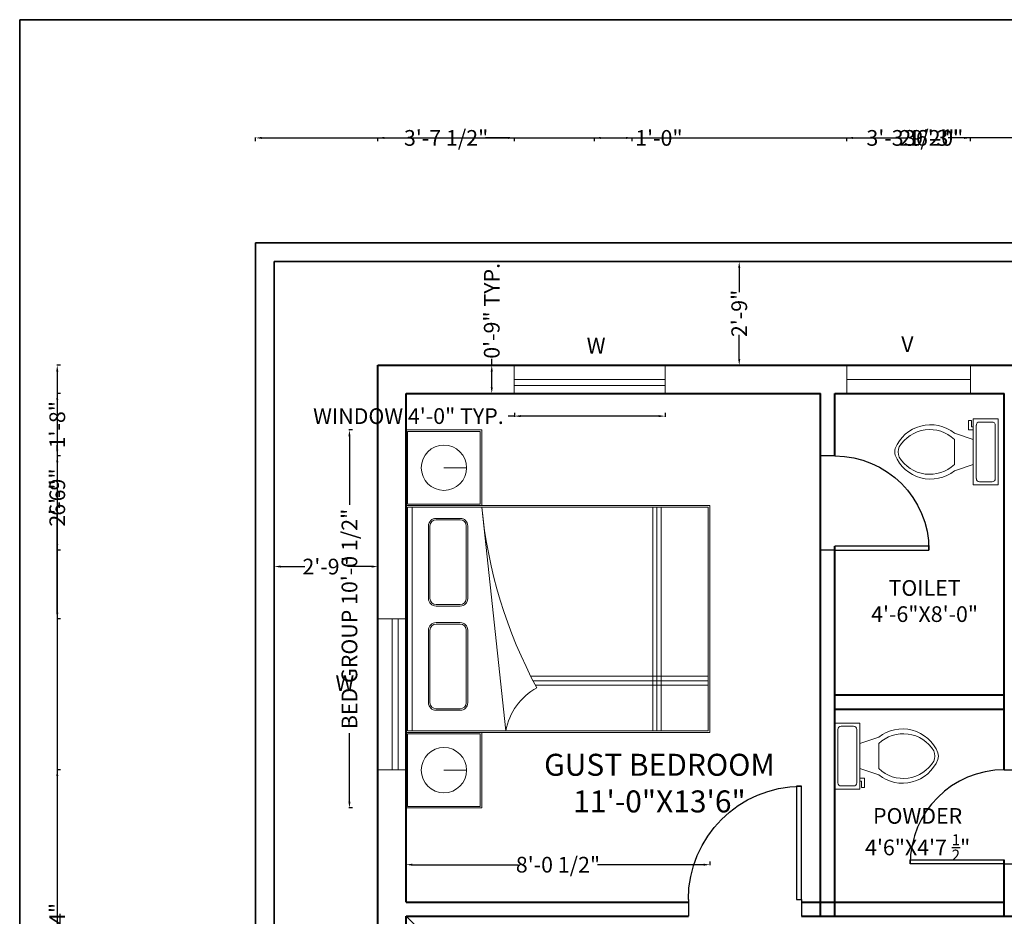
# Model space of a CAD drawing. Units: inches. Extents: x -231 to 349, y -511 to 252.
# Tile 5 of 6: x -231 to 82, y -33 to 252. Entities that reach past the tile are written whole.
import ezdxf

# ---------------------------------------------------------------- set-up
doc = ezdxf.new("R2010")
doc.units = ezdxf.units.IN
doc.header["$MEASUREMENT"] = 0
for name, color, linetype, lineweight in [('A-ANNO-DIMS', 7, 'Continuous', 18), ('A-ANNO-TEXT', 7, 'Continuous', 18), ('A-ANNO-TTLB', 7, 'Continuous', 35), ('A-AREA-IDEN', 7, 'Continuous', 25), ('A-FLOR-FIXT', 8, 'Continuous', 18), ('A-FLOR-STRS', 7, 'Continuous', 20), ('A-GLAZ', 177, 'Continuous', 20), ('A-WALL', 7, 'Continuous', 40), ('BED', 30, 'Continuous', 18), ('C-PROP', 7, 'Continuous', 35), ('DOOR', 42, 'Continuous', 25)]:
    doc.layers.add(name, color=color, linetype=linetype, lineweight=lineweight)
doc.styles.get("Standard").update_dxf_attribs({"font": 'arial.ttf'})
doc.dimstyles.get("Standard").update_dxf_attribs({"dimtxt": 5, "dimasz": 2, "dimexe": 0.18, "dimexo": 0.0625, "dimgap": 0.09, "dimtad": 0, "dimzin": 0, "dimdsep": 46, "dimlunit": 4, "dimtxsty": 'Standard', "dimcen": 0.09, "dimadec": 0, "dimazin": 0, "dimtfac": 1, "dimtofl": 0, "dimtmove": 0, "dimatfit": 3, "dimfxl": 1, "dimfxlon": 1, "dimtolj": 1, "dimtzin": 0, "dimarcsym": 0})

# ---------------------------------------------------------------- blocks, each defined once
blk = doc.blocks.new('*U2')
for p, q in [((0, 0), (0, -6)), ((40, 0), (40, -6))]:
    blk.add_line(p, q)
blk.add_lwpolyline([(0, 0), (0, 40), (1.75, 40), (1.75, 0)], close=True)
blk.add_arc((0, 0), 40, 0, 90)
blk = doc.blocks.new('A$C0EA4476A')
at = {"linetype": 'ByBlock', "lineweight": -2}
for p, q in [((0, 2.008), (0, 1.508)), ((0.5, 2.008), (0, 2.008)), ((0.01, 1.998), (0.01, 1.518)), ((0.49, 1.998), (0.01, 1.998)), ((0.49, 1.518), (0.49, 1.998)), ((0.5, 2.008), (2, 2.008)), ((0.5, 0), (0.5, 2.008)), ((0.5, 1.508), (0.5, 2.008)), ((0.51, 1.998), (1.99, 1.998)), ((0.51, 0.01), (0.51, 1.998)), ((0.51, 1.968), (1.99, 1.968)), ((1.99, 1.998), (1.99, 0.01)), ((2, 2.008), (2, 0)), ((2, 2.008), (2.5, 2.008)), ((2, 1.508), (2, 2.008)), ((2.01, 1.998), (2.49, 1.998)), ((2.01, 1.518), (2.01, 1.998)), ((2.49, 1.998), (2.49, 1.518)), ((2.5, 2.008), (2.5, 1.508)), ((0.696, 1.8603), (1.176, 1.8603)), ((0.696, 1.8503), (1.176, 1.8503)), ((1.3855, 1.8603), (1.8655, 1.8603)), ((1.3855, 1.8503), (1.8655, 1.8503)), ((0.646, 1.6503), (0.646, 1.8103)), ((0.656, 1.6503), (0.656, 1.8103)), ((1.216, 1.8103), (1.216, 1.6503)), ((1.226, 1.8103), (1.226, 1.6503)), ((1.3355, 1.6503), (1.3355, 1.8103)), ((1.3455, 1.6503), (1.3455, 1.8103)), ((1.9055, 1.8103), (1.9055, 1.6503)), ((1.9155, 1.8103), (1.9155, 1.6503)), ((0.25, 1.758), (0.25, 1.608)), ((2.25, 1.758), (2.25, 1.608)), ((1.176, 1.6103), (0.696, 1.6103)), ((1.176, 1.6003), (0.696, 1.6003)), ((1.8655, 1.6103), (1.3855, 1.6103)), ((1.8655, 1.6003), (1.3855, 1.6003)), ((0, 1.508), (0.5, 1.508)), ((0.01, 1.518), (0.49, 1.518)), ((1.99, 1.508), (0.51, 1.3488)), ((2.5, 1.508), (2, 1.508)), ((2.49, 1.518), (2.01, 1.518)), ((0.8715, 1.1845), (0.8715, 0.01)), ((0.8115, 1.1534), (0.8115, 0.01)), ((0.8415, 1.1692), (0.8415, 0.01)), ((0.51, 0.3775), (1.99, 0.3775)), ((0.51, 0.3495), (1.99, 0.3495)), ((0.51, 0.3216), (1.99, 0.3216)), ((1.99, 0.01), (0.51, 0.01)), ((2, 0), (0.5, 0))]:
    blk.add_line(p, q, dxfattribs=at)
for centre in [(0.25, 1.758), (2.25, 1.758)]:
    blk.add_circle(centre, 0.15, dxfattribs=at)
for centre, radius, start, end in [((0.696, 1.8103), 0.05, 90, 180), ((0.696, 1.8103), 0.04, 90, 180), ((1.176, 1.8103), 0.05, 0, 90), ((1.176, 1.8103), 0.04, 0, 90), ((1.3855, 1.8103), 0.05, 90, 180), ((1.3855, 1.8103), 0.04, 90, 180), ((1.8655, 1.8103), 0.05, 0, 90), ((1.8655, 1.8103), 0.04, 0, 90), ((0.696, 1.6503), 0.05, 180, 270), ((0.696, 1.6503), 0.04, 180, 270), ((1.176, 1.6503), 0.04, 270, 0), ((1.176, 1.6503), 0.05, 270, 0), ((1.3855, 1.6503), 0.05, 180, 270), ((1.3855, 1.6503), 0.04, 180, 270), ((1.8655, 1.6503), 0.05, 270, 0), ((1.8655, 1.6503), 0.04, 270, 0), ((2.2933, -1.6357), 3.1583, 95.51042, 118.33991), ((0.4397, 0.9519), 0.4031, 28.46882, 79.95566)]:
    blk.add_arc(centre, radius, start, end, dxfattribs=at)
blk = doc.blocks.new('A$C1A706E3E')
blk.add_blockref('A$C0EA4476A', (0, 0))
blk = doc.blocks.new('*U9')
for p, q in [((9.5, -6), (9.5, -2)), ((-10, -8.5), (-8, -8.5)), ((-10, -9.5), (-10, -8.5)), ((-8, -8.5), (-8, -8)), ((-7, -8), (-7, -9.5)), ((-4, -8), (-6, -14)), ((4, -8), (6, -14)), ((-7, -9.5), (-10, -9.5)), ((4, -14), (-4, -14))]:
    blk.add_line(p, q)
blk.add_lwpolyline([(10.5, -8), (10.5, 0), (-10.5, 0), (-10.5, -8)], close=True)
for points in [[(-9.5, -2), (-9.5, -6)], [(8.5, -1), (-8.5, -1)], [(-8.5, -7), (8.5, -7)]]:
    blk.add_lwpolyline(points)
for centre, radius, start, end in [((-8.62, -1.88), 0.884, 81.8699, 188.1301), ((8.62, -1.88), 0.884, 351.8699, 98.1301), ((-8.62, -6.12), 0.884, 171.8699, 278.1301), ((8.62, -6.12), 0.884, 261.8699, 8.1301), ((3.52, -21.58), 12.17, 141.4691, 247.9714), ((4.2, -21.82), 11.33, 136.3677, 238.9468), ((-3.52, -21.58), 12.17, 292.0284, 38.5307), ((-4.2, -21.82), 11.33, 301.053, 43.6321), ((0, -27.88), 4, 245.7318, 294.2682), ((0, -29), 4, 254.8605, 285.1395)]:
    blk.add_arc(centre, radius, start, end)
blk = doc.blocks.new('*D18')
at = {"layer": 'A-ANNO-DIMS', "color": 0, "lineweight": -2, "transparency": 16777216}
for p, q in [((-150.08, 79.26), (-150.08, 78.08)), ((-117.08, 79.26), (-117.08, 78.08)), ((-148.08, 78.26), (-140.36, 78.26)), ((-119.08, 78.26), (-126.8, 78.26))]:
    blk.add_line(p, q, dxfattribs=at)
at = {"layer": 'A-ANNO-DIMS', "color": 0, "transparency": 16777216}
for points in [[(-148.08, 78.6), (-148.08, 77.93), (-150.08, 78.26)], [(-119.08, 78.6), (-119.08, 77.93), (-117.08, 78.26)]]:
    blk.add_solid(points, dxfattribs=at)
at = {"layer": 'Defpoints', "color": 0, "transparency": 16777216}
for p in [(-150.08, 95.64), (-117.08, 95.64), (-150.08, 78.26)]:
    blk.add_point(p, dxfattribs=at)
at = {"layer": 'A-ANNO-DIMS', "color": 0, "transparency": 16777216, "insert": (-133.58, 78.26), "char_height": 5, "attachment_point": 5}
blk.add_mtext('\\A1;2\'-9"', dxfattribs=at)
blk = doc.blocks.new('*D19')
at = {"layer": 'A-ANNO-DIMS', "color": 0, "lineweight": -2, "transparency": 16777216}
for p, q in [((-2, 175.38), (-2.18, 175.38)), ((-2, 173.38), (-2, 165.66)), ((-2, 144.38), (-2, 152.1)), ((-2, 142.38), (-2.18, 142.38))]:
    blk.add_line(p, q, dxfattribs=at)
at = {"layer": 'A-ANNO-DIMS', "color": 0, "transparency": 16777216}
for points in [[(-2.34, 173.38), (-1.67, 173.38), (-2, 175.38)], [(-2.34, 144.38), (-1.67, 144.38), (-2, 142.38)]]:
    blk.add_solid(points, dxfattribs=at)
at = {"layer": 'Defpoints', "color": 0, "transparency": 16777216}
for p in [(-2, 175.38), (-2, 175.38), (-2, 142.38)]:
    blk.add_point(p, dxfattribs=at)
at = {"layer": 'A-ANNO-DIMS', "color": 0, "transparency": 16777216, "insert": (-2, 158.88), "char_height": 5, "attachment_point": 5, "rotation": 90}
blk.add_mtext('\\A1;2\'-9"', dxfattribs=at)
blk = doc.blocks.new('WIN-48IN')
for p, q in [((224.92, -56.7), (233.92, -56.7)), ((227.42, -56.7), (227.42, -104.7)), ((229.42, -56.7), (229.42, -104.7)), ((224.92, -104.7), (233.92, -104.7))]:
    blk.add_line(p, q)
blk = doc.blocks.new('*D30')
at = {"layer": 'A-ANNO-DIMS', "color": 0, "lineweight": -2, "transparency": 16777216}
for p, q in [((-73.62, 126.18), (-75.62, 126.18)), ((-73.62, 127.18), (-73.62, 126)), ((-27.62, 126.18), (-71.62, 126.18)), ((-25.62, 127.18), (-25.62, 126))]:
    blk.add_line(p, q, dxfattribs=at)
at = {"layer": 'A-ANNO-DIMS', "color": 0, "transparency": 16777216}
for points in [[(-71.62, 126.51), (-71.62, 125.85), (-73.62, 126.18)], [(-27.62, 126.51), (-27.62, 125.85), (-25.62, 126.18)]]:
    blk.add_solid(points, dxfattribs=at)
at = {"layer": 'Defpoints', "color": 0, "transparency": 16777216}
for p in [(-73.62, 133.38), (-25.62, 133.38), (-73.62, 126.18)]:
    blk.add_point(p, dxfattribs=at)
at = {"layer": 'A-ANNO-DIMS', "color": 0, "transparency": 16777216, "insert": (-107.35, 126.18), "char_height": 5, "attachment_point": 5}
blk.add_mtext('\\A1;WINDOW 4\'-0" TYP.', dxfattribs=at)
blk = doc.blocks.new('*D31')
at = {"layer": 'A-ANNO-DIMS', "color": 0, "lineweight": -2, "transparency": 16777216}
for p, q in [((-80.82, 142.38), (-80.82, 144.38)), ((-79.82, 142.38), (-81, 142.38)), ((-80.82, 135.38), (-80.82, 140.38)), ((-79.82, 133.38), (-81, 133.38))]:
    blk.add_line(p, q, dxfattribs=at)
at = {"layer": 'A-ANNO-DIMS', "color": 0, "transparency": 16777216}
for points in [[(-81.16, 140.38), (-80.49, 140.38), (-80.82, 142.38)], [(-81.16, 135.38), (-80.49, 135.38), (-80.82, 133.38)]]:
    blk.add_solid(points, dxfattribs=at)
at = {"layer": 'Defpoints', "color": 0, "transparency": 16777216}
for p in [(-80.82, 142.38), (-73.62, 142.38), (-73.62, 133.38)]:
    blk.add_point(p, dxfattribs=at)
at = {"layer": 'A-ANNO-DIMS', "color": 0, "transparency": 16777216, "insert": (-80.82, 159.71), "char_height": 5, "attachment_point": 5, "rotation": 90}
blk.add_mtext('\\A1;0\'-9" TYP.', dxfattribs=at)
blk = doc.blocks.new('*D34')
at = {"layer": 'A-ANNO-DIMS', "color": 0, "lineweight": -2, "transparency": 16777216}
for p, q in [((-125.14, 121.77), (-126.32, 121.77)), ((-126.14, 119.77), (-126.14, 97.9)), ((-126.14, 3.38), (-126.14, 25.25)), ((-125.14, 1.38), (-126.32, 1.38))]:
    blk.add_line(p, q, dxfattribs=at)
at = {"layer": 'A-ANNO-DIMS', "color": 0, "transparency": 16777216}
for points in [[(-126.47, 119.77), (-125.81, 119.77), (-126.14, 121.77)], [(-126.47, 3.38), (-125.81, 3.38), (-126.14, 1.38)]]:
    blk.add_solid(points, dxfattribs=at)
at = {"layer": 'Defpoints', "color": 0, "transparency": 16777216}
for p in [(-126.14, 121.77), (-108.08, 121.77), (-108.08, 1.38)]:
    blk.add_point(p, dxfattribs=at)
at = {"layer": 'A-ANNO-DIMS', "color": 0, "transparency": 16777216, "insert": (-126.14, 61.57), "char_height": 5, "attachment_point": 5, "rotation": 90}
blk.add_mtext('\\A1;BED GROUP 10\'-0 1/2"', dxfattribs=at)
blk = doc.blocks.new('*D35')
at = {"layer": 'A-ANNO-DIMS', "color": 0, "lineweight": -2, "transparency": 16777216}
for p, q in [((-108.08, -15.68), (-108.08, -16.86)), ((-106.08, -16.68), (-72.29, -16.68)), ((-13.38, -16.68), (-47.16, -16.68)), ((-11.38, -15.68), (-11.38, -16.86))]:
    blk.add_line(p, q, dxfattribs=at)
at = {"layer": 'A-ANNO-DIMS', "color": 0, "transparency": 16777216}
for points in [[(-106.08, -16.35), (-106.08, -17.02), (-108.08, -16.68)], [(-13.38, -16.35), (-13.38, -17.02), (-11.38, -16.68)]]:
    blk.add_solid(points, dxfattribs=at)
at = {"layer": 'Defpoints', "color": 0, "transparency": 16777216}
for p in [(-108.08, 1.38), (-11.38, 1.38), (-108.08, -16.68)]:
    blk.add_point(p, dxfattribs=at)
at = {"layer": 'A-ANNO-DIMS', "color": 0, "transparency": 16777216, "insert": (-59.73, -16.68), "char_height": 5, "attachment_point": 5}
blk.add_mtext('\\A1;8\'-0 1/2"', dxfattribs=at)
blk = doc.blocks.new('*D44')
at = {"layer": 'A-ANNO-DIMS', "color": 0, "lineweight": -2, "transparency": 16777216}
for p, q in [((-156.08, 213.78), (-156.08, 214.96)), ((-154.08, 214.78), (51.24, 214.78)), ((273.92, 214.78), (68.6, 214.78)), ((275.92, 213.78), (275.92, 214.96))]:
    blk.add_line(p, q, dxfattribs=at)
at = {"layer": 'A-ANNO-DIMS', "color": 0, "transparency": 16777216}
for points in [[(-154.08, 215.11), (-154.08, 214.45), (-156.08, 214.78)], [(273.92, 215.11), (273.92, 214.45), (275.92, 214.78)]]:
    blk.add_solid(points, dxfattribs=at)
at = {"layer": 'Defpoints', "color": 0, "transparency": 16777216}
for p in [(275.92, 214.78), (-156.08, 181.38), (275.92, 181.38)]:
    blk.add_point(p, dxfattribs=at)
at = {"layer": 'A-ANNO-DIMS', "color": 0, "transparency": 16777216, "insert": (59.92, 214.78), "char_height": 5, "attachment_point": 5}
blk.add_mtext('\\A1;36\'-0"', dxfattribs=at)
blk = doc.blocks.new('*D46')
at = {"layer": 'A-ANNO-DIMS', "color": 0, "lineweight": -2, "transparency": 16777216}
for p, q in [((-117.08, 213.78), (-117.08, 214.96)), ((-115.08, 214.78), (49.7, 214.78)), ((231.92, 214.78), (67.14, 214.78)), ((233.92, 213.78), (233.92, 214.96))]:
    blk.add_line(p, q, dxfattribs=at)
at = {"layer": 'A-ANNO-DIMS', "color": 0, "transparency": 16777216}
for points in [[(-115.08, 215.11), (-115.08, 214.45), (-117.08, 214.78)], [(231.92, 215.11), (231.92, 214.45), (233.92, 214.78)]]:
    blk.add_solid(points, dxfattribs=at)
at = {"layer": 'Defpoints', "color": 0, "transparency": 16777216}
for p in [(233.92, 214.78), (-117.08, 142.38), (233.92, 142.38)]:
    blk.add_point(p, dxfattribs=at)
at = {"layer": 'A-ANNO-DIMS', "color": 0, "transparency": 16777216, "insert": (58.42, 214.78), "char_height": 5, "attachment_point": 5}
blk.add_mtext('\\A1;29\'-3"', dxfattribs=at)
blk = doc.blocks.new('*D47')
at = {"layer": 'A-ANNO-DIMS', "color": 0, "lineweight": -2, "transparency": 16777216}
for p, q in [((-218.19, 142.38), (-219.37, 142.38)), ((-219.19, 140.38), (-219.19, -87.44)), ((-219.19, -332.62), (-219.19, -104.8)), ((-218.19, -334.62), (-219.37, -334.62))]:
    blk.add_line(p, q, dxfattribs=at)
at = {"layer": 'A-ANNO-DIMS', "color": 0, "transparency": 16777216}
for points in [[(-219.53, 140.38), (-218.86, 140.38), (-219.19, 142.38)], [(-219.53, -332.62), (-218.86, -332.62), (-219.19, -334.62)]]:
    blk.add_solid(points, dxfattribs=at)
at = {"layer": 'Defpoints', "color": 0, "transparency": 16777216}
for p in [(-117.08, 142.38), (-219.19, -334.62), (-96.08, -334.62)]:
    blk.add_point(p, dxfattribs=at)
at = {"layer": 'A-ANNO-DIMS', "color": 0, "transparency": 16777216, "insert": (-219.19, -96.12), "char_height": 5, "attachment_point": 5, "rotation": 90}
blk.add_mtext('\\A1;39\'-9"', dxfattribs=at)
blk = doc.blocks.new('*D49')
at = {"layer": 'A-ANNO-DIMS', "color": 0, "lineweight": -2, "transparency": 16777216}
for p, q in [((-117.08, 213.78), (-117.08, 214.96)), ((-115.08, 214.78), (-107.91, 214.78)), ((-75.62, 214.78), (-82.79, 214.78)), ((-73.62, 213.78), (-73.62, 214.96))]:
    blk.add_line(p, q, dxfattribs=at)
at = {"layer": 'A-ANNO-DIMS', "color": 0, "transparency": 16777216}
for points in [[(-115.08, 215.11), (-115.08, 214.45), (-117.08, 214.78)], [(-75.62, 215.11), (-75.62, 214.45), (-73.62, 214.78)]]:
    blk.add_solid(points, dxfattribs=at)
at = {"layer": 'Defpoints', "color": 0, "transparency": 16777216}
for p in [(-73.62, 214.78), (-117.08, 142.38), (-73.62, 142.38)]:
    blk.add_point(p, dxfattribs=at)
at = {"layer": 'A-ANNO-DIMS', "color": 0, "transparency": 16777216, "insert": (-95.35, 214.78), "char_height": 5, "attachment_point": 5}
blk.add_mtext('\\A1;3\'-7 1/2"', dxfattribs=at)
blk = doc.blocks.new('*D50')
at = {"layer": 'A-ANNO-DIMS', "color": 0, "lineweight": -2, "transparency": 16777216}
for p, q in [((32.24, 213.78), (32.24, 214.96)), ((34.24, 214.78), (39.38, 214.78)), ((69.63, 214.78), (64.49, 214.78)), ((71.63, 213.78), (71.63, 214.96))]:
    blk.add_line(p, q, dxfattribs=at)
at = {"layer": 'A-ANNO-DIMS', "color": 0, "transparency": 16777216}
for points in [[(34.24, 215.11), (34.24, 214.45), (32.24, 214.78)], [(69.63, 215.11), (69.63, 214.45), (71.63, 214.78)]]:
    blk.add_solid(points, dxfattribs=at)
at = {"layer": 'Defpoints', "color": 0, "transparency": 16777216}
for p in [(71.63, 214.78), (32.24, 142.38), (71.63, 142.38)]:
    blk.add_point(p, dxfattribs=at)
at = {"layer": 'A-ANNO-DIMS', "color": 0, "transparency": 16777216, "insert": (51.93, 214.78), "char_height": 5, "attachment_point": 5}
blk.add_mtext('\\A1;3\'-3 1/2"', dxfattribs=at)
blk = doc.blocks.new('*D51')
at = {"layer": 'A-ANNO-DIMS', "color": 0, "lineweight": -2, "transparency": 16777216}
for p, q in [((28.42, -488.55), (28.42, -489.73)), ((32.24, -488.55), (32.24, -489.73)), ((26.42, -489.55), (24.42, -489.55)), ((34.24, -489.55), (36.24, -489.55))]:
    blk.add_line(p, q, dxfattribs=at)
at = {"layer": 'A-ANNO-DIMS', "color": 0, "transparency": 16777216}
for points in [[(26.42, -489.21), (26.42, -489.88), (28.42, -489.55)], [(34.24, -489.21), (34.24, -489.88), (32.24, -489.55)]]:
    blk.add_solid(points, dxfattribs=at)
at = {"layer": 'Defpoints', "color": 0, "transparency": 16777216}
for p in [(28.42, 133.38), (32.24, 133.38), (32.24, -489.55)]:
    blk.add_point(p, dxfattribs=at)
at = {"layer": 'A-ANNO-DIMS', "color": 0, "transparency": 16777216, "insert": (42.97, -489.55), "char_height": 5, "attachment_point": 5}
blk.add_mtext('\\A1;0\'-4"', dxfattribs=at)
blk = doc.blocks.new('*D52')
at = {"layer": 'A-ANNO-DIMS', "color": 0, "lineweight": -2, "transparency": 16777216}
for p, q in [((-218.19, 142.38), (-219.37, 142.38)), ((-219.19, 140.38), (-219.19, 108.73)), ((-219.19, 63.57), (-219.19, 95.23)), ((-218.19, 61.57), (-219.37, 61.57))]:
    blk.add_line(p, q, dxfattribs=at)
at = {"layer": 'A-ANNO-DIMS', "color": 0, "transparency": 16777216}
for points in [[(-219.53, 140.38), (-218.86, 140.38), (-219.19, 142.38)], [(-219.53, 63.57), (-218.86, 63.57), (-219.19, 61.57)]]:
    blk.add_solid(points, dxfattribs=at)
at = {"layer": 'Defpoints', "color": 0, "transparency": 16777216}
for p in [(-117.08, 142.38), (-219.19, 61.57), (-117.08, 61.57)]:
    blk.add_point(p, dxfattribs=at)
at = {"layer": 'A-ANNO-DIMS', "color": 0, "transparency": 16777216, "insert": (-219.19, 101.98), "char_height": 5, "attachment_point": 5, "rotation": 90}
blk.add_mtext('\\A1;6\'-9"', dxfattribs=at)
blk = doc.blocks.new('*D53')
at = {"layer": 'A-ANNO-DIMS', "color": 0, "lineweight": -2, "transparency": 16777216}
for p, q in [((-218.19, 13.57), (-219.37, 13.57)), ((-219.19, 11.57), (-219.19, -29.65)), ((-219.19, -84.36), (-219.19, -43.13)), ((-218.19, -86.36), (-219.37, -86.36))]:
    blk.add_line(p, q, dxfattribs=at)
at = {"layer": 'A-ANNO-DIMS', "color": 0, "transparency": 16777216}
for points in [[(-219.53, 11.57), (-218.86, 11.57), (-219.19, 13.57)], [(-219.53, -84.36), (-218.86, -84.36), (-219.19, -86.36)]]:
    blk.add_solid(points, dxfattribs=at)
at = {"layer": 'Defpoints', "color": 0, "transparency": 16777216}
for p in [(-117.08, 13.57), (-219.19, -86.36), (-117.08, -86.36)]:
    blk.add_point(p, dxfattribs=at)
at = {"layer": 'A-ANNO-DIMS', "color": 0, "transparency": 16777216, "insert": (-219.19, -36.39), "char_height": 5, "attachment_point": 5, "rotation": 90}
blk.add_mtext('\\A1;8\'-4"', dxfattribs=at)
blk = doc.blocks.new('*D59')
at = {"layer": 'A-ANNO-DIMS', "color": 0, "lineweight": -2, "transparency": 16777216}
for p, q in [((17.8, -488.55), (17.8, -489.73)), ((23.92, -488.55), (23.92, -489.73)), ((19.8, -489.55), (21.92, -489.55)), ((23.92, -489.55), (25.92, -489.55))]:
    blk.add_line(p, q, dxfattribs=at)
at = {"layer": 'A-ANNO-DIMS', "color": 0, "transparency": 16777216}
for points in [[(19.8, -489.21), (19.8, -489.88), (17.8, -489.55)], [(21.92, -489.21), (21.92, -489.88), (23.92, -489.55)]]:
    blk.add_solid(points, dxfattribs=at)
at = {"layer": 'Defpoints', "color": 0, "transparency": 16777216}
for p in [(17.8, -28.62), (23.92, -33.12), (23.92, -489.55)]:
    blk.add_point(p, dxfattribs=at)
at = {"layer": 'A-ANNO-DIMS', "color": 0, "transparency": 16777216, "insert": (32.66, -489.55), "char_height": 5, "attachment_point": 5}
blk.add_mtext('\\A1;0\'-6"', dxfattribs=at)
blk = doc.blocks.new('*D61')
at = {"layer": 'A-ANNO-DIMS', "color": 0, "lineweight": -2, "transparency": 16777216}
for p, q in [((-218.19, 113.5), (-219.37, 113.5)), ((-219.19, 111.5), (-219.19, 105.27)), ((-219.19, 85.5), (-219.19, 91.72)), ((-218.19, 83.5), (-219.37, 83.5))]:
    blk.add_line(p, q, dxfattribs=at)
at = {"layer": 'A-ANNO-DIMS', "color": 0, "transparency": 16777216}
for points in [[(-219.53, 111.5), (-218.86, 111.5), (-219.19, 113.5)], [(-219.53, 85.5), (-218.86, 85.5), (-219.19, 83.5)]]:
    blk.add_solid(points, dxfattribs=at)
at = {"layer": 'Defpoints', "color": 0, "transparency": 16777216}
for p in [(28.42, 113.5), (-219.19, 83.5), (28.42, 83.5)]:
    blk.add_point(p, dxfattribs=at)
at = {"layer": 'A-ANNO-DIMS', "color": 0, "transparency": 16777216, "insert": (-219.19, 98.5), "char_height": 5, "attachment_point": 5, "rotation": 90}
blk.add_mtext('\\A1;2\'-6"', dxfattribs=at)
blk = doc.blocks.new('*D62')
at = {"layer": 'A-ANNO-DIMS', "color": 0, "lineweight": -2, "transparency": 16777216}
for p, q in [((-218.19, 133.38), (-219.37, 133.38)), ((-219.19, 131.38), (-219.19, 129.94)), ((-219.19, 115.5), (-219.19, 116.94)), ((-218.19, 113.5), (-219.37, 113.5))]:
    blk.add_line(p, q, dxfattribs=at)
at = {"layer": 'A-ANNO-DIMS', "color": 0, "transparency": 16777216}
for points in [[(-219.53, 131.38), (-218.86, 131.38), (-219.19, 133.38)], [(-219.53, 115.5), (-218.86, 115.5), (-219.19, 113.5)]]:
    blk.add_solid(points, dxfattribs=at)
at = {"layer": 'Defpoints', "color": 0, "transparency": 16777216}
for p in [(28.42, 133.38), (-219.19, 113.5), (28.42, 113.5)]:
    blk.add_point(p, dxfattribs=at)
at = {"layer": 'A-ANNO-DIMS', "color": 0, "transparency": 16777216, "insert": (-219.19, 123.44), "char_height": 5, "attachment_point": 5, "rotation": 90}
blk.add_mtext('\\A1;1\'-8"', dxfattribs=at)
blk = doc.blocks.new('*D68')
at = {"layer": 'A-ANNO-DIMS', "color": 0, "lineweight": -2, "transparency": 16777216}
for p, q in [((-48.08, 213.78), (-48.08, 214.96)), ((-46.08, 214.78), (-38.08, 214.78)), ((-36.08, 213.78), (-36.08, 214.96)), ((-36.08, 214.78), (-34.08, 214.78))]:
    blk.add_line(p, q, dxfattribs=at)
at = {"layer": 'A-ANNO-DIMS', "color": 0, "transparency": 16777216}
for points in [[(-46.08, 215.11), (-46.08, 214.45), (-48.08, 214.78)], [(-38.08, 215.11), (-38.08, 214.45), (-36.08, 214.78)]]:
    blk.add_solid(points, dxfattribs=at)
at = {"layer": 'Defpoints', "color": 0, "transparency": 16777216}
for p in [(-36.08, 214.78), (-48.08, -177.12), (-36.08, -177.12)]:
    blk.add_point(p, dxfattribs=at)
at = {"layer": 'A-ANNO-DIMS', "color": 0, "transparency": 16777216, "insert": (-27.58, 214.78), "char_height": 5, "attachment_point": 5}
blk.add_mtext('\\A1;1\'-0"', dxfattribs=at)

msp = doc.modelspace()

# ---------------------------------------------------------------- linework, layer by layer
at = {"layer": 'A-ANNO-TTLB'}
msp.add_lwpolyline([(-231.158, 252.428), (348.864, 252.428), (348.864, -511.312), (-231.158, -511.312)], close=True, dxfattribs=at)
at = {"layer": 'A-FLOR-STRS'}
msp.add_line((-72.08, -69.12), (-108.08, -33.12), dxfattribs=at)
at = {"layer": 'A-GLAZ'}
for p, q in [((32.236, 142.38), (32.236, 133.38)), ((71.634, 142.38), (71.634, 133.38)), ((71.634, 137.88), (32.236, 137.88))]:
    msp.add_line(p, q, dxfattribs=at)
at = {"layer": 'A-WALL'}
for p, q in [((-117.08, 142.38), (233.92, 142.38)), ((-117.08, -186.12), (-117.08, 142.38)), ((-108.08, 133.38), (23.92, 133.38)), ((-108.08, -28.62), (-108.08, 133.38)), ((23.92, -33.12), (23.92, 133.38)), ((28.42, 133.38), (82.42, 133.38)), ((28.42, 113.495), (28.42, 133.38)), ((82.42, 13.543), (82.42, 133.38)), ((28.42, -33.12), (28.42, 84.808)), ((28.42, 37.38), (82.42, 37.38)), ((28.42, 32.88), (82.42, 32.88)), ((82.42, -33.12), (82.42, -15.145)), ((-108.08, -28.62), (-18.197, -28.62)), ((17.803, -28.62), (82.42, -28.62)), ((-108.08, -177.12), (-108.08, -33.12)), ((-108.08, -33.12), (-18.197, -33.12)), ((17.803, -33.12), (23.92, -33.12)), ((23.92, -33.12), (86.92, -33.12))]:
    msp.add_line(p, q, dxfattribs=at)
at = {"layer": 'C-PROP'}
for p, q in [((-156.08, 181.38), (275.92, 181.38)), ((-156.08, -394.62), (-156.08, 181.38)), ((-150.08, 175.38), (269.92, 175.38)), ((-150.08, -388.62), (-150.08, 175.38))]:
    msp.add_line(p, q, dxfattribs=at)

# ---------------------------------------------------------------- block references
at = {"layer": 'A-FLOR-FIXT'}
for p, rotation in [((80.506, 114.767), 270), ((28.42, 17.907), 89.99999999999999)]:
    msp.add_blockref('*U9', p, dxfattribs=dict(at, rotation=rotation))
at = {"layer": 'A-GLAZ'}
for p, rotation in [((-130.328, -91.54), 90.00000000000003), ((116.839, -43.129), 180)]:
    msp.add_blockref('WIN-48IN', p, dxfattribs=dict(at, rotation=rotation))
at = {"layer": 'BED', "xscale": 48.15846712609579, "yscale": 48.15846712609579, "zscale": 48.15846712609579, "rotation": 90}
msp.add_blockref('A$C1A706E3E', (-11.378, 1.376), dxfattribs=at)
at = {"layer": 'DOOR', "yscale": 0.75, "zscale": 0.75}
for p, xscale, rotation in [((28.42, 83.495), -0.75, 270), ((82.42, -16.457), 0.75, 90.00000000000003)]:
    msp.add_blockref('*U2', p, dxfattribs=dict(at, xscale=xscale, rotation=rotation))
at = {"layer": 'DOOR', "xscale": -0.9, "yscale": 0.9, "zscale": 0.9}
msp.add_blockref('*U2', (17.803, -27.72), dxfattribs=at)

# ---------------------------------------------------------------- texts
at = {"layer": 'A-ANNO-TEXT', "char_height": 5, "attachment_point": 1}
for s, insert in [('\\A1;W', (-50.574, 151.115)), ('\\A1;V', (49.591, 151.603)), ('\\A1;W', (-130.597, 43.673))]:
    msp.add_mtext_dynamic_manual_height_columns(s, width=7.82759, gutter_width=1, heights=[0], dxfattribs=dict(at, insert=insert))
at = {"layer": 'A-AREA-IDEN', "attachment_point": 1}
for s, insert, char_height in [('\\A1;\\pxqc;TOILET\\P4\'-6"X8\'-0"', (5.698, 73.957), 5), ('\\pxqc;GUST BEDROOM\\P11\'-0"X13\'6"', (-78.739, 18.637), 7), ('\\A1;\\pxqc;POWDER\\P4\'6"X4\'7 {\\H0.7x;\\S1/2;}"', (3.484, 1.356), 5)]:
    msp.add_mtext_dynamic_manual_height_columns(s, width=102.65834, gutter_width=1, heights=[0], dxfattribs=dict(at, insert=insert, char_height=char_height))

# ---------------------------------------------------------------- dimensions: what is measured, and where the dimension line sits
at = {"layer": 'A-ANNO-DIMS'}
for base, p1, p2, override, picture, middle in [((-73.624, 214.78), (-117.08, 142.38), (-73.624, 142.38), {"dimdec": 1, "dimlfac": 1, "dimrnd": 0, "dimzin": 1, "dimdsep": 46, "dimlunit": 4, "dimfrac": 2}, '*D49', (-95.352, 214.78)), ((71.634, 214.78), (32.236, 142.38), (71.634, 142.38), {"dimdec": 1, "dimlfac": 1, "dimrnd": 0, "dimzin": 1, "dimdsep": 46, "dimlunit": 4, "dimfrac": 2}, '*D50', (51.935, 214.78)), ((275.92, 214.78), (-156.08, 181.38), (275.92, 181.38), {"dimdec": 1, "dimlfac": 1, "dimrnd": 0, "dimzin": 1, "dimdsep": 46, "dimlunit": 4, "dimfrac": 2}, '*D44', (59.92, 214.78)), ((233.92, 214.78), (-117.08, 142.38), (233.92, 142.38), {"dimdec": 1, "dimlfac": 1, "dimrnd": 0, "dimzin": 1, "dimdsep": 46, "dimlunit": 4, "dimfrac": 2}, '*D46', (58.42, 214.78)), ((-36.08, 214.78), (-48.08, -177.12), (-36.08, -177.12), {"dimdec": 1, "dimlfac": 1, "dimrnd": 0, "dimzin": 1, "dimdsep": 46, "dimlunit": 4, "dimfrac": 2}, '*D68', (-27.58, 214.78)), ((32.236, -489.548), (28.42, 133.38), (32.236, 133.38), {"dimdec": 1, "dimlfac": 1, "dimrnd": 0, "dimzin": 1, "dimdsep": 46, "dimlunit": 4, "dimfrac": 2}, '*D51', (42.971, -489.548)), ((-150.08, 78.265), (-117.08, 95.639), (-150.08, 95.639), {"dimclrd": 0, "dimclre": 0, "dimclrt": 0}, '*D18', (-133.58, 78.265)), ((23.92, -489.548), (17.803, -28.62), (23.92, -33.12), {"dimdec": 1, "dimlfac": 1, "dimrnd": 0, "dimzin": 1, "dimdsep": 46, "dimlunit": 4, "dimfrac": 2}, '*D59', (32.655, -489.548))]:
    dim = msp.add_linear_dim(base=base, p1=p1, p2=p2, dimstyle='Standard', override=override, dxfattribs=at)
    dim.commit()
    dim.dimension.update_dxf_attribs({"geometry": picture, "text_midpoint": middle})
for base, p1, p2, angle, text, picture, middle in [((-80.824, 142.38), (-73.624, 133.38), (-73.624, 142.38), 90, '<> TYP.', '*D31', (-80.824, 159.708)), ((-73.624, 126.18), (-25.624, 133.38), (-73.624, 133.38), 180, 'WINDOW <> TYP.', '*D30', (-107.35, 126.18)), ((-126.14, 121.773), (-108.08, 1.376), (-108.08, 121.773), 90, 'BED GROUP <>', '*D34', (-126.14, 61.574))]:
    dim = msp.add_linear_dim(base=base, p1=p1, p2=p2, angle=angle, text=text, dimstyle='Standard', override={"dimdec": 1, "dimlfac": 1, "dimrnd": 0, "dimzin": 1, "dimdsep": 46, "dimlunit": 4, "dimfrac": 2}, dxfattribs=at)
    dim.commit()
    dim.dimension.update_dxf_attribs({"geometry": picture, "text_midpoint": middle})
for base, p1, p2, angle, override, picture, middle in [((-2.002, 175.38), (-2.002, 142.38), (-2.002, 175.38), 90, {"dimclrd": 0, "dimclre": 0, "dimclrt": 0}, '*D19', (-2.002, 158.88)), ((-219.195, -334.62), (-117.08, 142.38), (-96.08, -334.62), 90, {"dimdec": 1, "dimlfac": 1, "dimrnd": 0, "dimzin": 1, "dimdsep": 46, "dimlunit": 4, "dimfrac": 2}, '*D47', (-219.195, -96.12)), ((-219.195, 61.574), (-117.08, 142.38), (-117.08, 61.574), 90, {"dimdec": 1, "dimlfac": 1, "dimrnd": 0, "dimzin": 1, "dimdsep": 46, "dimlunit": 4, "dimfrac": 2}, '*D52', (-219.195, 101.977)), ((-219.195, 113.495), (28.42, 133.38), (28.42, 113.495), 90, {"dimdec": 1, "dimlfac": 1, "dimrnd": 0, "dimzin": 1, "dimdsep": 46, "dimlunit": 4, "dimfrac": 2}, '*D62', (-219.195, 123.437)), ((-219.195, 83.495), (28.42, 113.495), (28.42, 83.495), 90, {"dimdec": 1, "dimlfac": 1, "dimrnd": 0, "dimzin": 1, "dimdsep": 46, "dimlunit": 4, "dimfrac": 2}, '*D61', (-219.195, 98.495)), ((-219.195, -86.359), (-117.08, 13.574), (-117.08, -86.359), 90, {"dimdec": 1, "dimlfac": 1, "dimrnd": 0, "dimzin": 1, "dimdsep": 46, "dimlunit": 4, "dimfrac": 2}, '*D53', (-219.195, -36.392)), ((-108.08, -16.683), (-11.378, 1.376), (-108.08, 1.376), 180, {"dimdec": 1, "dimlfac": 1, "dimrnd": 0, "dimzin": 1, "dimdsep": 46, "dimlunit": 4, "dimfrac": 2}, '*D35', (-59.729, -16.683))]:
    dim = msp.add_linear_dim(base=base, p1=p1, p2=p2, angle=angle, dimstyle='Standard', override=override, dxfattribs=at)
    dim.commit()
    dim.dimension.update_dxf_attribs({"geometry": picture, "text_midpoint": middle})

doc.saveas('drawing.dxf')
